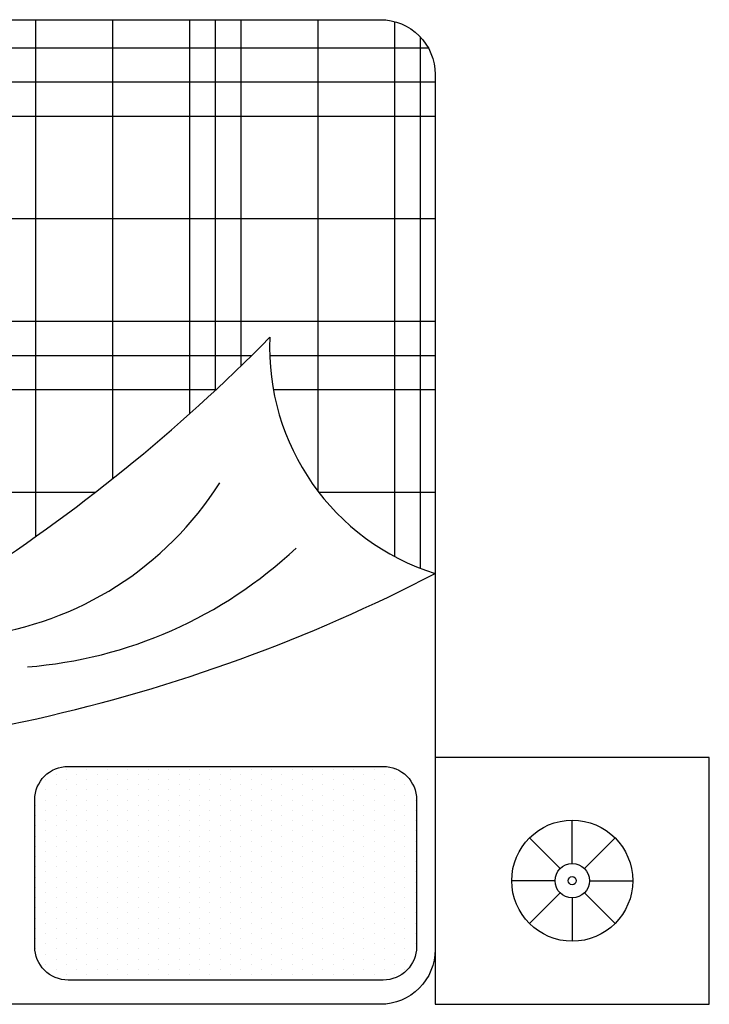
# Model space of a CAD drawing. Units: millimetres. Extents: x 2817 to 5038, y 1110 to 3565.
# Tile 21 of 21: x 4992 to 5038, y 3499 to 3565. Entities that reach past the tile are written whole.
import ezdxf

# ---------------------------------------------------------------- set-up
doc = ezdxf.new("R2010")
doc.units = ezdxf.units.MM
doc.layers.add('BLOCK', color=6, linetype='Continuous')
doc.layers.add('FURNITURE', color=219, linetype='Continuous', lineweight=18)

# ---------------------------------------------------------------- blocks, each defined once
blk = doc.blocks.new('*X7')
at = {"color": 0}
for p, q in [((276.598, 451.25), (280.51, 451.25)), ((275.455, 450.625), (280.51, 450.625)), ((274.411, 450), (280.51, 450)), ((265.51, 448.125), (267.634, 448.125)), ((271.723, 448.125), (280.51, 448.125)), ((265.51, 446.25), (268.465, 446.25)), ((269.519, 446.25), (280.51, 446.25)), ((265.51, 445.625), (268.531, 445.625)), ((268.866, 445.625), (280.51, 445.625)), ((265.51, 445), (280.51, 445)), ((265.51, 443.125), (280.51, 443.125)), ((265.51, 441.25), (280.51, 441.25)), ((265.51, 440.625), (280.51, 440.625)), ((265.634, 440), (280.386, 440))]:
    blk.add_line(p, q, dxfattribs=at)
blk = doc.blocks.new('*X8')
at = {"color": 0}
for p, q in [((280.312, 439.886), (280.312, 452.896)), ((278.906, 439.482), (278.906, 452.338)), ((277.5, 439.482), (277.5, 451.702)), ((277.031, 439.482), (277.031, 451.471)), ((276.562, 439.482), (276.562, 451.231)), ((275.156, 439.482), (275.156, 450.451)), ((265.781, 439.797), (265.781, 449.511)), ((273.75, 439.482), (273.75, 449.576)), ((266.25, 439.517), (266.25, 449.296)), ((273.281, 439.482), (273.281, 449.261)), ((272.812, 439.482), (272.812, 448.934)), ((267.656, 439.482), (267.656, 448.095)), ((271.406, 439.482), (271.406, 447.876)), ((270, 439.482), (270, 446.689)), ((269.531, 439.482), (269.531, 446.262)), ((269.062, 439.482), (269.062, 445.817))]:
    blk.add_line(p, q, dxfattribs=at)
blk = doc.blocks.new('*X9')
at = {"color": 0}
for p, q in [((266.4375, 457.03125), (266.4375, 457.03125)), ((266.8125, 457.03125), (266.8125, 457.03125)), ((267.1875, 457.03125), (267.1875, 457.03125)), ((267.5625, 457.03125), (267.5625, 457.03125)), ((267.9375, 457.03125), (267.9375, 457.03125)), ((268.3125, 457.03125), (268.3125, 457.03125)), ((268.6875, 457.03125), (268.6875, 457.03125)), ((269.0625, 457.03125), (269.0625, 457.03125)), ((269.4375, 457.03125), (269.4375, 457.03125)), ((269.8125, 457.03125), (269.8125, 457.03125)), ((270.1875, 457.03125), (270.1875, 457.03125)), ((270.5625, 457.03125), (270.5625, 457.03125)), ((270.9375, 457.03125), (270.9375, 457.03125)), ((271.3125, 457.03125), (271.3125, 457.03125)), ((271.6875, 457.03125), (271.6875, 457.03125)), ((272.0625, 457.03125), (272.0625, 457.03125)), ((266.0625, 456.84375), (266.0625, 456.84375)), ((266.25, 456.9375), (266.25, 456.9375)), ((266.4375, 456.84375), (266.4375, 456.84375)), ((266.625, 456.9375), (266.625, 456.9375)), ((266.8125, 456.84375), (266.8125, 456.84375)), ((267, 456.9375), (267, 456.9375)), ((267.1875, 456.84375), (267.1875, 456.84375)), ((267.375, 456.9375), (267.375, 456.9375)), ((267.5625, 456.84375), (267.5625, 456.84375)), ((267.75, 456.9375), (267.75, 456.9375)), ((267.9375, 456.84375), (267.9375, 456.84375)), ((268.125, 456.9375), (268.125, 456.9375)), ((268.3125, 456.84375), (268.3125, 456.84375)), ((268.5, 456.9375), (268.5, 456.9375)), ((268.6875, 456.84375), (268.6875, 456.84375)), ((268.875, 456.9375), (268.875, 456.9375)), ((269.0625, 456.84375), (269.0625, 456.84375)), ((269.25, 456.9375), (269.25, 456.9375)), ((269.4375, 456.84375), (269.4375, 456.84375)), ((269.625, 456.9375), (269.625, 456.9375)), ((269.8125, 456.84375), (269.8125, 456.84375)), ((270, 456.9375), (270, 456.9375)), ((270.1875, 456.84375), (270.1875, 456.84375)), ((270.375, 456.9375), (270.375, 456.9375)), ((270.5625, 456.84375), (270.5625, 456.84375)), ((270.75, 456.9375), (270.75, 456.9375)), ((270.9375, 456.84375), (270.9375, 456.84375)), ((271.125, 456.9375), (271.125, 456.9375)), ((271.3125, 456.84375), (271.3125, 456.84375)), ((271.5, 456.9375), (271.5, 456.9375)), ((271.6875, 456.84375), (271.6875, 456.84375)), ((271.875, 456.9375), (271.875, 456.9375)), ((272.0625, 456.84375), (272.0625, 456.84375)), ((272.25, 456.9375), (272.25, 456.9375)), ((272.4375, 456.84375), (272.4375, 456.84375)), ((266.25, 456.75), (266.25, 456.75)), ((266.625, 456.75), (266.625, 456.75)), ((267, 456.75), (267, 456.75)), ((267.375, 456.75), (267.375, 456.75)), ((267.75, 456.75), (267.75, 456.75)), ((268.125, 456.75), (268.125, 456.75)), ((268.5, 456.75), (268.5, 456.75)), ((268.875, 456.75), (268.875, 456.75)), ((269.25, 456.75), (269.25, 456.75)), ((269.625, 456.75), (269.625, 456.75)), ((270, 456.75), (270, 456.75)), ((270.375, 456.75), (270.375, 456.75)), ((270.75, 456.75), (270.75, 456.75)), ((271.125, 456.75), (271.125, 456.75)), ((271.5, 456.75), (271.5, 456.75)), ((271.875, 456.75), (271.875, 456.75)), ((272.25, 456.75), (272.25, 456.75)), ((272.625, 456.75), (272.625, 456.75)), ((265.875, 456.5625), (265.875, 456.5625)), ((266.0625, 456.65625), (266.0625, 456.65625)), ((266.25, 456.5625), (266.25, 456.5625)), ((266.4375, 456.65625), (266.4375, 456.65625)), ((266.625, 456.5625), (266.625, 456.5625)), ((266.8125, 456.65625), (266.8125, 456.65625)), ((267, 456.5625), (267, 456.5625)), ((267.1875, 456.65625), (267.1875, 456.65625)), ((267.375, 456.5625), (267.375, 456.5625)), ((267.5625, 456.65625), (267.5625, 456.65625)), ((267.75, 456.5625), (267.75, 456.5625)), ((267.9375, 456.65625), (267.9375, 456.65625)), ((268.125, 456.5625), (268.125, 456.5625)), ((268.3125, 456.65625), (268.3125, 456.65625)), ((268.5, 456.5625), (268.5, 456.5625)), ((268.6875, 456.65625), (268.6875, 456.65625)), ((268.875, 456.5625), (268.875, 456.5625)), ((269.0625, 456.65625), (269.0625, 456.65625)), ((269.25, 456.5625), (269.25, 456.5625)), ((269.4375, 456.65625), (269.4375, 456.65625)), ((269.625, 456.5625), (269.625, 456.5625)), ((269.8125, 456.65625), (269.8125, 456.65625)), ((270, 456.5625), (270, 456.5625)), ((270.1875, 456.65625), (270.1875, 456.65625)), ((270.375, 456.5625), (270.375, 456.5625)), ((270.5625, 456.65625), (270.5625, 456.65625)), ((270.75, 456.5625), (270.75, 456.5625)), ((270.9375, 456.65625), (270.9375, 456.65625)), ((271.125, 456.5625), (271.125, 456.5625)), ((271.3125, 456.65625), (271.3125, 456.65625)), ((271.5, 456.5625), (271.5, 456.5625)), ((271.6875, 456.65625), (271.6875, 456.65625)), ((271.875, 456.5625), (271.875, 456.5625)), ((272.0625, 456.65625), (272.0625, 456.65625)), ((272.25, 456.5625), (272.25, 456.5625)), ((272.4375, 456.65625), (272.4375, 456.65625)), ((272.625, 456.5625), (272.625, 456.5625)), ((265.875, 456.375), (265.875, 456.375)), ((266.0625, 456.46875), (266.0625, 456.46875)), ((266.25, 456.375), (266.25, 456.375)), ((266.4375, 456.46875), (266.4375, 456.46875)), ((266.625, 456.375), (266.625, 456.375)), ((266.8125, 456.46875), (266.8125, 456.46875)), ((267, 456.375), (267, 456.375)), ((267.1875, 456.46875), (267.1875, 456.46875)), ((267.375, 456.375), (267.375, 456.375)), ((267.5625, 456.46875), (267.5625, 456.46875)), ((267.75, 456.375), (267.75, 456.375)), ((267.9375, 456.46875), (267.9375, 456.46875)), ((268.125, 456.375), (268.125, 456.375)), ((268.3125, 456.46875), (268.3125, 456.46875)), ((268.5, 456.375), (268.5, 456.375)), ((268.6875, 456.46875), (268.6875, 456.46875)), ((268.875, 456.375), (268.875, 456.375)), ((269.0625, 456.46875), (269.0625, 456.46875)), ((269.25, 456.375), (269.25, 456.375)), ((269.4375, 456.46875), (269.4375, 456.46875)), ((269.625, 456.375), (269.625, 456.375)), ((269.8125, 456.46875), (269.8125, 456.46875)), ((270, 456.375), (270, 456.375)), ((270.1875, 456.46875), (270.1875, 456.46875)), ((270.375, 456.375), (270.375, 456.375)), ((270.5625, 456.46875), (270.5625, 456.46875)), ((270.75, 456.375), (270.75, 456.375)), ((270.9375, 456.46875), (270.9375, 456.46875)), ((271.125, 456.375), (271.125, 456.375)), ((271.3125, 456.46875), (271.3125, 456.46875)), ((271.5, 456.375), (271.5, 456.375)), ((271.6875, 456.46875), (271.6875, 456.46875)), ((271.875, 456.375), (271.875, 456.375)), ((272.0625, 456.46875), (272.0625, 456.46875)), ((272.25, 456.375), (272.25, 456.375)), ((272.4375, 456.46875), (272.4375, 456.46875)), ((272.625, 456.375), (272.625, 456.375)), ((272.8125, 456.46875), (272.8125, 456.46875)), ((265.875, 456.1875), (265.875, 456.1875)), ((266.0625, 456.28125), (266.0625, 456.28125)), ((266.25, 456.1875), (266.25, 456.1875)), ((266.4375, 456.28125), (266.4375, 456.28125)), ((266.625, 456.1875), (266.625, 456.1875)), ((266.8125, 456.28125), (266.8125, 456.28125)), ((267, 456.1875), (267, 456.1875)), ((267.1875, 456.28125), (267.1875, 456.28125)), ((267.375, 456.1875), (267.375, 456.1875)), ((267.5625, 456.28125), (267.5625, 456.28125)), ((267.75, 456.1875), (267.75, 456.1875)), ((267.9375, 456.28125), (267.9375, 456.28125)), ((268.125, 456.1875), (268.125, 456.1875)), ((268.3125, 456.28125), (268.3125, 456.28125)), ((268.5, 456.1875), (268.5, 456.1875)), ((268.6875, 456.28125), (268.6875, 456.28125)), ((268.875, 456.1875), (268.875, 456.1875)), ((269.0625, 456.28125), (269.0625, 456.28125)), ((269.25, 456.1875), (269.25, 456.1875)), ((269.4375, 456.28125), (269.4375, 456.28125)), ((269.625, 456.1875), (269.625, 456.1875)), ((269.8125, 456.28125), (269.8125, 456.28125)), ((270, 456.1875), (270, 456.1875)), ((270.1875, 456.28125), (270.1875, 456.28125)), ((270.375, 456.1875), (270.375, 456.1875)), ((270.5625, 456.28125), (270.5625, 456.28125)), ((270.75, 456.1875), (270.75, 456.1875)), ((270.9375, 456.28125), (270.9375, 456.28125)), ((271.125, 456.1875), (271.125, 456.1875)), ((271.3125, 456.28125), (271.3125, 456.28125)), ((271.5, 456.1875), (271.5, 456.1875)), ((271.6875, 456.28125), (271.6875, 456.28125)), ((271.875, 456.1875), (271.875, 456.1875)), ((272.0625, 456.28125), (272.0625, 456.28125)), ((272.25, 456.1875), (272.25, 456.1875)), ((272.4375, 456.28125), (272.4375, 456.28125)), ((272.625, 456.1875), (272.625, 456.1875)), ((272.8125, 456.28125), (272.8125, 456.28125)), ((265.875, 456), (265.875, 456)), ((266.0625, 456.09375), (266.0625, 456.09375)), ((266.25, 456), (266.25, 456)), ((266.4375, 456.09375), (266.4375, 456.09375)), ((266.625, 456), (266.625, 456)), ((266.8125, 456.09375), (266.8125, 456.09375)), ((267, 456), (267, 456)), ((267.1875, 456.09375), (267.1875, 456.09375)), ((267.375, 456), (267.375, 456)), ((267.5625, 456.09375), (267.5625, 456.09375)), ((267.75, 456), (267.75, 456)), ((267.9375, 456.09375), (267.9375, 456.09375)), ((268.125, 456), (268.125, 456)), ((268.3125, 456.09375), (268.3125, 456.09375)), ((268.5, 456), (268.5, 456)), ((268.6875, 456.09375), (268.6875, 456.09375)), ((268.875, 456), (268.875, 456)), ((269.0625, 456.09375), (269.0625, 456.09375)), ((269.25, 456), (269.25, 456)), ((269.4375, 456.09375), (269.4375, 456.09375)), ((269.625, 456), (269.625, 456)), ((269.8125, 456.09375), (269.8125, 456.09375)), ((270, 456), (270, 456)), ((270.1875, 456.09375), (270.1875, 456.09375)), ((270.375, 456), (270.375, 456)), ((270.5625, 456.09375), (270.5625, 456.09375)), ((270.75, 456), (270.75, 456)), ((270.9375, 456.09375), (270.9375, 456.09375)), ((271.125, 456), (271.125, 456)), ((271.3125, 456.09375), (271.3125, 456.09375)), ((271.5, 456), (271.5, 456)), ((271.6875, 456.09375), (271.6875, 456.09375)), ((271.875, 456), (271.875, 456)), ((272.0625, 456.09375), (272.0625, 456.09375)), ((272.25, 456), (272.25, 456)), ((272.4375, 456.09375), (272.4375, 456.09375)), ((272.625, 456), (272.625, 456)), ((272.8125, 456.09375), (272.8125, 456.09375)), ((265.875, 455.8125), (265.875, 455.8125)), ((266.0625, 455.90625), (266.0625, 455.90625)), ((266.25, 455.8125), (266.25, 455.8125)), ((266.4375, 455.90625), (266.4375, 455.90625)), ((266.625, 455.8125), (266.625, 455.8125)), ((266.8125, 455.90625), (266.8125, 455.90625)), ((267, 455.8125), (267, 455.8125)), ((267.1875, 455.90625), (267.1875, 455.90625)), ((267.375, 455.8125), (267.375, 455.8125)), ((267.5625, 455.90625), (267.5625, 455.90625)), ((267.75, 455.8125), (267.75, 455.8125)), ((267.9375, 455.90625), (267.9375, 455.90625)), ((268.125, 455.8125), (268.125, 455.8125)), ((268.3125, 455.90625), (268.3125, 455.90625)), ((268.5, 455.8125), (268.5, 455.8125)), ((268.6875, 455.90625), (268.6875, 455.90625)), ((268.875, 455.8125), (268.875, 455.8125)), ((269.0625, 455.90625), (269.0625, 455.90625)), ((269.25, 455.8125), (269.25, 455.8125)), ((269.4375, 455.90625), (269.4375, 455.90625)), ((269.625, 455.8125), (269.625, 455.8125)), ((269.8125, 455.90625), (269.8125, 455.90625)), ((270, 455.8125), (270, 455.8125)), ((270.1875, 455.90625), (270.1875, 455.90625)), ((270.375, 455.8125), (270.375, 455.8125)), ((270.5625, 455.90625), (270.5625, 455.90625)), ((270.75, 455.8125), (270.75, 455.8125)), ((270.9375, 455.90625), (270.9375, 455.90625)), ((271.125, 455.8125), (271.125, 455.8125)), ((271.3125, 455.90625), (271.3125, 455.90625)), ((271.5, 455.8125), (271.5, 455.8125)), ((271.6875, 455.90625), (271.6875, 455.90625)), ((271.875, 455.8125), (271.875, 455.8125)), ((272.0625, 455.90625), (272.0625, 455.90625)), ((272.25, 455.8125), (272.25, 455.8125)), ((272.4375, 455.90625), (272.4375, 455.90625)), ((272.625, 455.8125), (272.625, 455.8125)), ((272.8125, 455.90625), (272.8125, 455.90625)), ((265.875, 455.625), (265.875, 455.625)), ((266.0625, 455.71875), (266.0625, 455.71875)), ((266.25, 455.625), (266.25, 455.625)), ((266.4375, 455.71875), (266.4375, 455.71875)), ((266.625, 455.625), (266.625, 455.625)), ((266.8125, 455.71875), (266.8125, 455.71875)), ((267, 455.625), (267, 455.625)), ((267.1875, 455.71875), (267.1875, 455.71875)), ((267.375, 455.625), (267.375, 455.625)), ((267.5625, 455.71875), (267.5625, 455.71875)), ((267.75, 455.625), (267.75, 455.625)), ((267.9375, 455.71875), (267.9375, 455.71875)), ((268.125, 455.625), (268.125, 455.625)), ((268.3125, 455.71875), (268.3125, 455.71875)), ((268.5, 455.625), (268.5, 455.625)), ((268.6875, 455.71875), (268.6875, 455.71875)), ((268.875, 455.625), (268.875, 455.625)), ((269.0625, 455.71875), (269.0625, 455.71875)), ((269.25, 455.625), (269.25, 455.625)), ((269.4375, 455.71875), (269.4375, 455.71875)), ((269.625, 455.625), (269.625, 455.625)), ((269.8125, 455.71875), (269.8125, 455.71875)), ((270, 455.625), (270, 455.625)), ((270.1875, 455.71875), (270.1875, 455.71875)), ((270.375, 455.625), (270.375, 455.625)), ((270.5625, 455.71875), (270.5625, 455.71875)), ((270.75, 455.625), (270.75, 455.625)), ((270.9375, 455.71875), (270.9375, 455.71875)), ((271.125, 455.625), (271.125, 455.625)), ((271.3125, 455.71875), (271.3125, 455.71875)), ((271.5, 455.625), (271.5, 455.625)), ((271.6875, 455.71875), (271.6875, 455.71875)), ((271.875, 455.625), (271.875, 455.625)), ((272.0625, 455.71875), (272.0625, 455.71875)), ((272.25, 455.625), (272.25, 455.625)), ((272.4375, 455.71875), (272.4375, 455.71875)), ((272.625, 455.625), (272.625, 455.625)), ((272.8125, 455.71875), (272.8125, 455.71875)), ((265.875, 455.4375), (265.875, 455.4375)), ((266.0625, 455.53125), (266.0625, 455.53125)), ((266.25, 455.4375), (266.25, 455.4375)), ((266.4375, 455.53125), (266.4375, 455.53125)), ((266.625, 455.4375), (266.625, 455.4375)), ((266.8125, 455.53125), (266.8125, 455.53125)), ((267, 455.4375), (267, 455.4375)), ((267.1875, 455.53125), (267.1875, 455.53125)), ((267.375, 455.4375), (267.375, 455.4375)), ((267.5625, 455.53125), (267.5625, 455.53125)), ((267.75, 455.4375), (267.75, 455.4375)), ((267.9375, 455.53125), (267.9375, 455.53125)), ((268.125, 455.4375), (268.125, 455.4375)), ((268.3125, 455.53125), (268.3125, 455.53125)), ((268.5, 455.4375), (268.5, 455.4375)), ((268.6875, 455.53125), (268.6875, 455.53125)), ((268.875, 455.4375), (268.875, 455.4375)), ((269.0625, 455.53125), (269.0625, 455.53125)), ((269.25, 455.4375), (269.25, 455.4375)), ((269.4375, 455.53125), (269.4375, 455.53125)), ((269.625, 455.4375), (269.625, 455.4375)), ((269.8125, 455.53125), (269.8125, 455.53125)), ((270, 455.4375), (270, 455.4375)), ((270.1875, 455.53125), (270.1875, 455.53125)), ((270.375, 455.4375), (270.375, 455.4375)), ((270.5625, 455.53125), (270.5625, 455.53125)), ((270.75, 455.4375), (270.75, 455.4375)), ((270.9375, 455.53125), (270.9375, 455.53125)), ((271.125, 455.4375), (271.125, 455.4375)), ((271.3125, 455.53125), (271.3125, 455.53125)), ((271.5, 455.4375), (271.5, 455.4375)), ((271.6875, 455.53125), (271.6875, 455.53125)), ((271.875, 455.4375), (271.875, 455.4375)), ((272.0625, 455.53125), (272.0625, 455.53125)), ((272.25, 455.4375), (272.25, 455.4375)), ((272.4375, 455.53125), (272.4375, 455.53125)), ((272.625, 455.4375), (272.625, 455.4375)), ((272.8125, 455.53125), (272.8125, 455.53125)), ((265.875, 455.25), (265.875, 455.25)), ((266.0625, 455.34375), (266.0625, 455.34375)), ((266.25, 455.25), (266.25, 455.25)), ((266.4375, 455.34375), (266.4375, 455.34375)), ((266.625, 455.25), (266.625, 455.25)), ((266.8125, 455.34375), (266.8125, 455.34375)), ((267, 455.25), (267, 455.25)), ((267.1875, 455.34375), (267.1875, 455.34375)), ((267.375, 455.25), (267.375, 455.25)), ((267.5625, 455.34375), (267.5625, 455.34375)), ((267.75, 455.25), (267.75, 455.25)), ((267.9375, 455.34375), (267.9375, 455.34375)), ((268.125, 455.25), (268.125, 455.25)), ((268.3125, 455.34375), (268.3125, 455.34375)), ((268.5, 455.25), (268.5, 455.25)), ((268.6875, 455.34375), (268.6875, 455.34375)), ((268.875, 455.25), (268.875, 455.25)), ((269.0625, 455.34375), (269.0625, 455.34375)), ((269.25, 455.25), (269.25, 455.25)), ((269.4375, 455.34375), (269.4375, 455.34375)), ((269.625, 455.25), (269.625, 455.25)), ((269.8125, 455.34375), (269.8125, 455.34375)), ((270, 455.25), (270, 455.25)), ((270.1875, 455.34375), (270.1875, 455.34375)), ((270.375, 455.25), (270.375, 455.25)), ((270.5625, 455.34375), (270.5625, 455.34375)), ((270.75, 455.25), (270.75, 455.25)), ((270.9375, 455.34375), (270.9375, 455.34375)), ((271.125, 455.25), (271.125, 455.25)), ((271.3125, 455.34375), (271.3125, 455.34375)), ((271.5, 455.25), (271.5, 455.25)), ((271.6875, 455.34375), (271.6875, 455.34375)), ((271.875, 455.25), (271.875, 455.25)), ((272.0625, 455.34375), (272.0625, 455.34375)), ((272.25, 455.25), (272.25, 455.25)), ((272.4375, 455.34375), (272.4375, 455.34375)), ((272.625, 455.25), (272.625, 455.25)), ((272.8125, 455.34375), (272.8125, 455.34375)), ((265.875, 455.0625), (265.875, 455.0625)), ((266.0625, 455.15625), (266.0625, 455.15625)), ((266.25, 455.0625), (266.25, 455.0625)), ((266.4375, 455.15625), (266.4375, 455.15625)), ((266.625, 455.0625), (266.625, 455.0625)), ((266.8125, 455.15625), (266.8125, 455.15625)), ((267, 455.0625), (267, 455.0625)), ((267.1875, 455.15625), (267.1875, 455.15625)), ((267.375, 455.0625), (267.375, 455.0625)), ((267.5625, 455.15625), (267.5625, 455.15625)), ((267.75, 455.0625), (267.75, 455.0625)), ((267.9375, 455.15625), (267.9375, 455.15625)), ((268.125, 455.0625), (268.125, 455.0625)), ((268.3125, 455.15625), (268.3125, 455.15625)), ((268.5, 455.0625), (268.5, 455.0625)), ((268.6875, 455.15625), (268.6875, 455.15625)), ((268.875, 455.0625), (268.875, 455.0625)), ((269.0625, 455.15625), (269.0625, 455.15625)), ((269.25, 455.0625), (269.25, 455.0625)), ((269.4375, 455.15625), (269.4375, 455.15625)), ((269.625, 455.0625), (269.625, 455.0625)), ((269.8125, 455.15625), (269.8125, 455.15625)), ((270, 455.0625), (270, 455.0625)), ((270.1875, 455.15625), (270.1875, 455.15625)), ((270.375, 455.0625), (270.375, 455.0625)), ((270.5625, 455.15625), (270.5625, 455.15625)), ((270.75, 455.0625), (270.75, 455.0625)), ((270.9375, 455.15625), (270.9375, 455.15625)), ((271.125, 455.0625), (271.125, 455.0625)), ((271.3125, 455.15625), (271.3125, 455.15625)), ((271.5, 455.0625), (271.5, 455.0625)), ((271.6875, 455.15625), (271.6875, 455.15625)), ((271.875, 455.0625), (271.875, 455.0625)), ((272.0625, 455.15625), (272.0625, 455.15625)), ((272.25, 455.0625), (272.25, 455.0625)), ((272.4375, 455.15625), (272.4375, 455.15625)), ((272.625, 455.0625), (272.625, 455.0625)), ((272.8125, 455.15625), (272.8125, 455.15625)), ((265.875, 454.875), (265.875, 454.875)), ((266.0625, 454.96875), (266.0625, 454.96875)), ((266.25, 454.875), (266.25, 454.875)), ((266.4375, 454.96875), (266.4375, 454.96875)), ((266.625, 454.875), (266.625, 454.875)), ((266.8125, 454.96875), (266.8125, 454.96875)), ((267, 454.875), (267, 454.875)), ((267.1875, 454.96875), (267.1875, 454.96875)), ((267.375, 454.875), (267.375, 454.875)), ((267.5625, 454.96875), (267.5625, 454.96875)), ((267.75, 454.875), (267.75, 454.875)), ((267.9375, 454.96875), (267.9375, 454.96875)), ((268.125, 454.875), (268.125, 454.875)), ((268.3125, 454.96875), (268.3125, 454.96875)), ((268.5, 454.875), (268.5, 454.875)), ((268.6875, 454.96875), (268.6875, 454.96875)), ((268.875, 454.875), (268.875, 454.875)), ((269.0625, 454.96875), (269.0625, 454.96875)), ((269.25, 454.875), (269.25, 454.875)), ((269.4375, 454.96875), (269.4375, 454.96875)), ((269.625, 454.875), (269.625, 454.875)), ((269.8125, 454.96875), (269.8125, 454.96875)), ((270, 454.875), (270, 454.875)), ((270.1875, 454.96875), (270.1875, 454.96875)), ((270.375, 454.875), (270.375, 454.875)), ((270.5625, 454.96875), (270.5625, 454.96875)), ((270.75, 454.875), (270.75, 454.875)), ((270.9375, 454.96875), (270.9375, 454.96875)), ((271.125, 454.875), (271.125, 454.875)), ((271.3125, 454.96875), (271.3125, 454.96875)), ((271.5, 454.875), (271.5, 454.875)), ((271.6875, 454.96875), (271.6875, 454.96875)), ((271.875, 454.875), (271.875, 454.875)), ((272.0625, 454.96875), (272.0625, 454.96875)), ((272.25, 454.875), (272.25, 454.875)), ((272.4375, 454.96875), (272.4375, 454.96875)), ((272.625, 454.875), (272.625, 454.875)), ((272.8125, 454.96875), (272.8125, 454.96875)), ((265.875, 454.6875), (265.875, 454.6875)), ((266.0625, 454.78125), (266.0625, 454.78125)), ((266.25, 454.6875), (266.25, 454.6875)), ((266.4375, 454.78125), (266.4375, 454.78125)), ((266.625, 454.6875), (266.625, 454.6875)), ((266.8125, 454.78125), (266.8125, 454.78125)), ((267, 454.6875), (267, 454.6875)), ((267.1875, 454.78125), (267.1875, 454.78125)), ((267.375, 454.6875), (267.375, 454.6875)), ((267.5625, 454.78125), (267.5625, 454.78125)), ((267.75, 454.6875), (267.75, 454.6875)), ((267.9375, 454.78125), (267.9375, 454.78125)), ((268.125, 454.6875), (268.125, 454.6875)), ((268.3125, 454.78125), (268.3125, 454.78125)), ((268.5, 454.6875), (268.5, 454.6875)), ((268.6875, 454.78125), (268.6875, 454.78125)), ((268.875, 454.6875), (268.875, 454.6875)), ((269.0625, 454.78125), (269.0625, 454.78125)), ((269.25, 454.6875), (269.25, 454.6875)), ((269.4375, 454.78125), (269.4375, 454.78125)), ((269.625, 454.6875), (269.625, 454.6875)), ((269.8125, 454.78125), (269.8125, 454.78125)), ((270, 454.6875), (270, 454.6875)), ((270.1875, 454.78125), (270.1875, 454.78125)), ((270.375, 454.6875), (270.375, 454.6875)), ((270.5625, 454.78125), (270.5625, 454.78125)), ((270.75, 454.6875), (270.75, 454.6875)), ((270.9375, 454.78125), (270.9375, 454.78125)), ((271.125, 454.6875), (271.125, 454.6875)), ((271.3125, 454.78125), (271.3125, 454.78125)), ((271.5, 454.6875), (271.5, 454.6875)), ((271.6875, 454.78125), (271.6875, 454.78125)), ((271.875, 454.6875), (271.875, 454.6875)), ((272.0625, 454.78125), (272.0625, 454.78125)), ((272.25, 454.6875), (272.25, 454.6875)), ((272.4375, 454.78125), (272.4375, 454.78125)), ((272.625, 454.6875), (272.625, 454.6875)), ((272.8125, 454.78125), (272.8125, 454.78125)), ((266.0625, 454.59375), (266.0625, 454.59375)), ((266.4375, 454.59375), (266.4375, 454.59375)), ((266.8125, 454.59375), (266.8125, 454.59375)), ((267.1875, 454.59375), (267.1875, 454.59375)), ((267.5625, 454.59375), (267.5625, 454.59375)), ((267.9375, 454.59375), (267.9375, 454.59375)), ((268.3125, 454.59375), (268.3125, 454.59375)), ((268.6875, 454.59375), (268.6875, 454.59375)), ((269.0625, 454.59375), (269.0625, 454.59375)), ((269.4375, 454.59375), (269.4375, 454.59375)), ((269.8125, 454.59375), (269.8125, 454.59375)), ((270.1875, 454.59375), (270.1875, 454.59375)), ((270.5625, 454.59375), (270.5625, 454.59375)), ((270.9375, 454.59375), (270.9375, 454.59375)), ((271.3125, 454.59375), (271.3125, 454.59375)), ((271.6875, 454.59375), (271.6875, 454.59375)), ((272.0625, 454.59375), (272.0625, 454.59375)), ((272.4375, 454.59375), (272.4375, 454.59375)), ((272.8125, 454.59375), (272.8125, 454.59375)), ((265.875, 454.5), (265.875, 454.5)), ((266.0625, 454.40625), (266.0625, 454.40625)), ((266.25, 454.5), (266.25, 454.5)), ((266.4375, 454.40625), (266.4375, 454.40625)), ((266.625, 454.5), (266.625, 454.5)), ((266.8125, 454.40625), (266.8125, 454.40625)), ((267, 454.5), (267, 454.5)), ((267.1875, 454.40625), (267.1875, 454.40625)), ((267.375, 454.5), (267.375, 454.5)), ((267.5625, 454.40625), (267.5625, 454.40625)), ((267.75, 454.5), (267.75, 454.5)), ((267.9375, 454.40625), (267.9375, 454.40625)), ((268.125, 454.5), (268.125, 454.5)), ((268.3125, 454.40625), (268.3125, 454.40625)), ((268.5, 454.5), (268.5, 454.5)), ((268.6875, 454.40625), (268.6875, 454.40625)), ((268.875, 454.5), (268.875, 454.5)), ((269.0625, 454.40625), (269.0625, 454.40625)), ((269.25, 454.5), (269.25, 454.5)), ((269.4375, 454.40625), (269.4375, 454.40625)), ((269.625, 454.5), (269.625, 454.5)), ((269.8125, 454.40625), (269.8125, 454.40625)), ((270, 454.5), (270, 454.5)), ((270.1875, 454.40625), (270.1875, 454.40625)), ((270.375, 454.5), (270.375, 454.5)), ((270.5625, 454.40625), (270.5625, 454.40625)), ((270.75, 454.5), (270.75, 454.5)), ((270.9375, 454.40625), (270.9375, 454.40625)), ((271.125, 454.5), (271.125, 454.5)), ((271.3125, 454.40625), (271.3125, 454.40625)), ((271.5, 454.5), (271.5, 454.5)), ((271.6875, 454.40625), (271.6875, 454.40625)), ((271.875, 454.5), (271.875, 454.5)), ((272.0625, 454.40625), (272.0625, 454.40625)), ((272.25, 454.5), (272.25, 454.5)), ((272.4375, 454.40625), (272.4375, 454.40625)), ((272.625, 454.5), (272.625, 454.5)), ((272.8125, 454.40625), (272.8125, 454.40625)), ((265.875, 454.3125), (265.875, 454.3125)), ((266.0625, 454.21875), (266.0625, 454.21875)), ((266.25, 454.3125), (266.25, 454.3125)), ((266.4375, 454.21875), (266.4375, 454.21875)), ((266.625, 454.3125), (266.625, 454.3125)), ((266.8125, 454.21875), (266.8125, 454.21875)), ((267, 454.3125), (267, 454.3125)), ((267.1875, 454.21875), (267.1875, 454.21875)), ((267.375, 454.3125), (267.375, 454.3125)), ((267.5625, 454.21875), (267.5625, 454.21875)), ((267.75, 454.3125), (267.75, 454.3125)), ((267.9375, 454.21875), (267.9375, 454.21875)), ((268.125, 454.3125), (268.125, 454.3125)), ((268.3125, 454.21875), (268.3125, 454.21875)), ((268.5, 454.3125), (268.5, 454.3125)), ((268.6875, 454.21875), (268.6875, 454.21875)), ((268.875, 454.3125), (268.875, 454.3125)), ((269.0625, 454.21875), (269.0625, 454.21875)), ((269.25, 454.3125), (269.25, 454.3125)), ((269.4375, 454.21875), (269.4375, 454.21875)), ((269.625, 454.3125), (269.625, 454.3125)), ((269.8125, 454.21875), (269.8125, 454.21875)), ((270, 454.3125), (270, 454.3125)), ((270.1875, 454.21875), (270.1875, 454.21875)), ((270.375, 454.3125), (270.375, 454.3125)), ((270.5625, 454.21875), (270.5625, 454.21875)), ((270.75, 454.3125), (270.75, 454.3125)), ((270.9375, 454.21875), (270.9375, 454.21875)), ((271.125, 454.3125), (271.125, 454.3125)), ((271.3125, 454.21875), (271.3125, 454.21875)), ((271.5, 454.3125), (271.5, 454.3125)), ((271.6875, 454.21875), (271.6875, 454.21875)), ((271.875, 454.3125), (271.875, 454.3125)), ((272.0625, 454.21875), (272.0625, 454.21875)), ((272.25, 454.3125), (272.25, 454.3125)), ((272.4375, 454.21875), (272.4375, 454.21875)), ((272.625, 454.3125), (272.625, 454.3125)), ((272.8125, 454.21875), (272.8125, 454.21875)), ((265.875, 454.125), (265.875, 454.125)), ((266.0625, 454.03125), (266.0625, 454.03125)), ((266.25, 454.125), (266.25, 454.125)), ((266.4375, 454.03125), (266.4375, 454.03125)), ((266.625, 454.125), (266.625, 454.125)), ((266.8125, 454.03125), (266.8125, 454.03125)), ((267, 454.125), (267, 454.125)), ((267.1875, 454.03125), (267.1875, 454.03125)), ((267.375, 454.125), (267.375, 454.125)), ((267.5625, 454.03125), (267.5625, 454.03125)), ((267.75, 454.125), (267.75, 454.125)), ((267.9375, 454.03125), (267.9375, 454.03125)), ((268.125, 454.125), (268.125, 454.125)), ((268.3125, 454.03125), (268.3125, 454.03125)), ((268.5, 454.125), (268.5, 454.125)), ((268.6875, 454.03125), (268.6875, 454.03125)), ((268.875, 454.125), (268.875, 454.125)), ((269.0625, 454.03125), (269.0625, 454.03125)), ((269.25, 454.125), (269.25, 454.125)), ((269.4375, 454.03125), (269.4375, 454.03125)), ((269.625, 454.125), (269.625, 454.125)), ((269.8125, 454.03125), (269.8125, 454.03125)), ((270, 454.125), (270, 454.125)), ((270.1875, 454.03125), (270.1875, 454.03125)), ((270.375, 454.125), (270.375, 454.125)), ((270.5625, 454.03125), (270.5625, 454.03125)), ((270.75, 454.125), (270.75, 454.125)), ((270.9375, 454.03125), (270.9375, 454.03125)), ((271.125, 454.125), (271.125, 454.125)), ((271.3125, 454.03125), (271.3125, 454.03125)), ((271.5, 454.125), (271.5, 454.125)), ((271.6875, 454.03125), (271.6875, 454.03125)), ((271.875, 454.125), (271.875, 454.125)), ((272.0625, 454.03125), (272.0625, 454.03125)), ((272.25, 454.125), (272.25, 454.125)), ((272.4375, 454.03125), (272.4375, 454.03125)), ((272.625, 454.125), (272.625, 454.125)), ((272.8125, 454.03125), (272.8125, 454.03125)), ((265.875, 453.9375), (265.875, 453.9375)), ((266.0625, 453.84375), (266.0625, 453.84375)), ((266.25, 453.9375), (266.25, 453.9375)), ((266.4375, 453.84375), (266.4375, 453.84375)), ((266.625, 453.9375), (266.625, 453.9375)), ((266.8125, 453.84375), (266.8125, 453.84375)), ((267, 453.9375), (267, 453.9375)), ((267.1875, 453.84375), (267.1875, 453.84375)), ((267.375, 453.9375), (267.375, 453.9375)), ((267.5625, 453.84375), (267.5625, 453.84375)), ((267.75, 453.9375), (267.75, 453.9375)), ((267.9375, 453.84375), (267.9375, 453.84375)), ((268.125, 453.9375), (268.125, 453.9375)), ((268.3125, 453.84375), (268.3125, 453.84375)), ((268.5, 453.9375), (268.5, 453.9375)), ((268.6875, 453.84375), (268.6875, 453.84375)), ((268.875, 453.9375), (268.875, 453.9375)), ((269.0625, 453.84375), (269.0625, 453.84375)), ((269.25, 453.9375), (269.25, 453.9375)), ((269.4375, 453.84375), (269.4375, 453.84375)), ((269.625, 453.9375), (269.625, 453.9375)), ((269.8125, 453.84375), (269.8125, 453.84375)), ((270, 453.9375), (270, 453.9375)), ((270.1875, 453.84375), (270.1875, 453.84375)), ((270.375, 453.9375), (270.375, 453.9375)), ((270.5625, 453.84375), (270.5625, 453.84375)), ((270.75, 453.9375), (270.75, 453.9375)), ((270.9375, 453.84375), (270.9375, 453.84375)), ((271.125, 453.9375), (271.125, 453.9375)), ((271.3125, 453.84375), (271.3125, 453.84375)), ((271.5, 453.9375), (271.5, 453.9375)), ((271.6875, 453.84375), (271.6875, 453.84375)), ((271.875, 453.9375), (271.875, 453.9375)), ((272.0625, 453.84375), (272.0625, 453.84375)), ((272.25, 453.9375), (272.25, 453.9375)), ((272.4375, 453.84375), (272.4375, 453.84375)), ((272.625, 453.9375), (272.625, 453.9375)), ((272.8125, 453.84375), (272.8125, 453.84375)), ((265.875, 453.75), (265.875, 453.75)), ((266.0625, 453.65625), (266.0625, 453.65625)), ((266.25, 453.75), (266.25, 453.75)), ((266.4375, 453.65625), (266.4375, 453.65625)), ((266.625, 453.75), (266.625, 453.75)), ((266.8125, 453.65625), (266.8125, 453.65625)), ((267, 453.75), (267, 453.75)), ((267.1875, 453.65625), (267.1875, 453.65625)), ((267.375, 453.75), (267.375, 453.75)), ((267.5625, 453.65625), (267.5625, 453.65625)), ((267.75, 453.75), (267.75, 453.75)), ((267.9375, 453.65625), (267.9375, 453.65625)), ((268.125, 453.75), (268.125, 453.75)), ((268.3125, 453.65625), (268.3125, 453.65625)), ((268.5, 453.75), (268.5, 453.75)), ((268.6875, 453.65625), (268.6875, 453.65625)), ((268.875, 453.75), (268.875, 453.75)), ((269.0625, 453.65625), (269.0625, 453.65625)), ((269.25, 453.75), (269.25, 453.75)), ((269.4375, 453.65625), (269.4375, 453.65625)), ((269.625, 453.75), (269.625, 453.75)), ((269.8125, 453.65625), (269.8125, 453.65625)), ((270, 453.75), (270, 453.75)), ((270.1875, 453.65625), (270.1875, 453.65625)), ((270.375, 453.75), (270.375, 453.75)), ((270.5625, 453.65625), (270.5625, 453.65625)), ((270.75, 453.75), (270.75, 453.75)), ((270.9375, 453.65625), (270.9375, 453.65625)), ((271.125, 453.75), (271.125, 453.75)), ((271.3125, 453.65625), (271.3125, 453.65625)), ((271.5, 453.75), (271.5, 453.75)), ((271.6875, 453.65625), (271.6875, 453.65625)), ((271.875, 453.75), (271.875, 453.75)), ((272.0625, 453.65625), (272.0625, 453.65625)), ((272.25, 453.75), (272.25, 453.75)), ((272.4375, 453.65625), (272.4375, 453.65625)), ((272.625, 453.75), (272.625, 453.75)), ((272.8125, 453.65625), (272.8125, 453.65625)), ((266.0625, 453.46875), (266.0625, 453.46875)), ((266.25, 453.5625), (266.25, 453.5625)), ((266.4375, 453.46875), (266.4375, 453.46875)), ((266.625, 453.5625), (266.625, 453.5625)), ((266.8125, 453.46875), (266.8125, 453.46875)), ((267, 453.5625), (267, 453.5625)), ((267.1875, 453.46875), (267.1875, 453.46875)), ((267.375, 453.5625), (267.375, 453.5625)), ((267.5625, 453.46875), (267.5625, 453.46875)), ((267.75, 453.5625), (267.75, 453.5625)), ((267.9375, 453.46875), (267.9375, 453.46875)), ((268.125, 453.5625), (268.125, 453.5625)), ((268.3125, 453.46875), (268.3125, 453.46875)), ((268.5, 453.5625), (268.5, 453.5625)), ((268.6875, 453.46875), (268.6875, 453.46875)), ((268.875, 453.5625), (268.875, 453.5625)), ((269.0625, 453.46875), (269.0625, 453.46875)), ((269.25, 453.5625), (269.25, 453.5625)), ((269.4375, 453.46875), (269.4375, 453.46875)), ((269.625, 453.5625), (269.625, 453.5625)), ((269.8125, 453.46875), (269.8125, 453.46875)), ((270, 453.5625), (270, 453.5625)), ((270.1875, 453.46875), (270.1875, 453.46875)), ((270.375, 453.5625), (270.375, 453.5625)), ((270.5625, 453.46875), (270.5625, 453.46875)), ((270.75, 453.5625), (270.75, 453.5625)), ((270.9375, 453.46875), (270.9375, 453.46875)), ((271.125, 453.5625), (271.125, 453.5625)), ((271.3125, 453.46875), (271.3125, 453.46875)), ((271.5, 453.5625), (271.5, 453.5625)), ((271.6875, 453.46875), (271.6875, 453.46875)), ((271.875, 453.5625), (271.875, 453.5625)), ((272.0625, 453.46875), (272.0625, 453.46875)), ((272.25, 453.5625), (272.25, 453.5625)), ((272.4375, 453.46875), (272.4375, 453.46875)), ((272.625, 453.5625), (272.625, 453.5625)), ((266.0625, 453.28125), (266.0625, 453.28125)), ((266.25, 453.375), (266.25, 453.375)), ((266.4375, 453.28125), (266.4375, 453.28125)), ((266.625, 453.375), (266.625, 453.375)), ((266.8125, 453.28125), (266.8125, 453.28125)), ((267, 453.375), (267, 453.375)), ((267.1875, 453.28125), (267.1875, 453.28125)), ((267.375, 453.375), (267.375, 453.375)), ((267.5625, 453.28125), (267.5625, 453.28125)), ((267.75, 453.375), (267.75, 453.375)), ((267.9375, 453.28125), (267.9375, 453.28125)), ((268.125, 453.375), (268.125, 453.375)), ((268.3125, 453.28125), (268.3125, 453.28125)), ((268.5, 453.375), (268.5, 453.375)), ((268.6875, 453.28125), (268.6875, 453.28125)), ((268.875, 453.375), (268.875, 453.375)), ((269.0625, 453.28125), (269.0625, 453.28125)), ((269.25, 453.375), (269.25, 453.375)), ((269.4375, 453.28125), (269.4375, 453.28125)), ((269.625, 453.375), (269.625, 453.375)), ((269.8125, 453.28125), (269.8125, 453.28125)), ((270, 453.375), (270, 453.375)), ((270.1875, 453.28125), (270.1875, 453.28125)), ((270.375, 453.375), (270.375, 453.375)), ((270.5625, 453.28125), (270.5625, 453.28125)), ((270.75, 453.375), (270.75, 453.375)), ((270.9375, 453.28125), (270.9375, 453.28125)), ((271.125, 453.375), (271.125, 453.375)), ((271.3125, 453.28125), (271.3125, 453.28125)), ((271.5, 453.375), (271.5, 453.375)), ((271.6875, 453.28125), (271.6875, 453.28125)), ((271.875, 453.375), (271.875, 453.375)), ((272.0625, 453.28125), (272.0625, 453.28125)), ((272.25, 453.375), (272.25, 453.375)), ((272.4375, 453.28125), (272.4375, 453.28125)), ((272.625, 453.375), (272.625, 453.375)), ((266.25, 453.1875), (266.25, 453.1875)), ((266.625, 453.1875), (266.625, 453.1875)), ((267, 453.1875), (267, 453.1875)), ((267.375, 453.1875), (267.375, 453.1875)), ((267.75, 453.1875), (267.75, 453.1875)), ((268.125, 453.1875), (268.125, 453.1875)), ((268.5, 453.1875), (268.5, 453.1875)), ((268.875, 453.1875), (268.875, 453.1875)), ((269.25, 453.1875), (269.25, 453.1875)), ((269.625, 453.1875), (269.625, 453.1875)), ((270, 453.1875), (270, 453.1875)), ((270.375, 453.1875), (270.375, 453.1875)), ((270.75, 453.1875), (270.75, 453.1875)), ((271.125, 453.1875), (271.125, 453.1875)), ((271.5, 453.1875), (271.5, 453.1875)), ((271.875, 453.1875), (271.875, 453.1875)), ((272.25, 453.1875), (272.25, 453.1875))]:
    blk.add_line(p, q, dxfattribs=at)
blk = doc.blocks.new('A$C52E67D0D')
at = {"layer": 'BLOCK'}
for p, q in [((250.5, 1605.5), (250.5, 1684.7)), ((228.3, 1596.3), (172.3, 1652.3)), ((272.7, 1596.3), (328.7, 1652.3)), ((219.1, 1574.1), (139.9, 1574.1)), ((281.9, 1574.1), (361.1, 1574.1)), ((228.3, 1551.9), (172.3, 1495.9)), ((272.7, 1551.9), (328.7, 1495.9)), ((250.5, 1542.8), (250.5, 1463.5))]:
    blk.add_line(p, q, dxfattribs=at)
for points in [[(1901, 0), (601, 0, -0.414214), (501, 100), (501, 1700, -0.414214), (601, 1800), (1901, 1800, -0.414214), (2001, 1700), (2001, 100, -0.414214)], [(1171.8, 1365.1), (595.8, 1365.1, -0.414214), (535, 1425.9), (535, 1694.8, -0.414214), (595.8, 1755.7), (1171.8, 1755.7, -0.414214), (1232.6, 1694.8), (1232.6, 1425.9, -0.414214)]]:
    blk.add_lwpolyline(points, format="xyb", close=True, dxfattribs=at)
blk.add_lwpolyline([(501, 1348.6), (501, 1799.6), (0, 1799.6), (0, 1348.6)], close=True, dxfattribs=at)
for radius in [110.6, 31.4, 7.46]:
    blk.add_circle((250.5, 1574.1), radius, dxfattribs=at)
for centre, radius, start, end in [((1888.6, -1664.5), 3015.3, 87.8642, 117.4001), ((3101, -1685.8), 3227.7, 109.926, 135.3977), ((1308.8, 377.9), 807.6, 94.4436, 133.2788), ((1410.8, 520.2), 610.8, 97.2157, 147.6656), ((371.4, 600.4), 432, 357.3792, 72.5379)]:
    blk.add_arc(centre, radius, start, end, dxfattribs=at)
at = {"layer": 'BLOCK', "xscale": 100, "yscale": 100, "zscale": 100}
for name in ['*X9', '*X8', '*X7']:
    blk.add_blockref(name, (-26050, -43948.2), dxfattribs=at)

msp = doc.modelspace()

# ---------------------------------------------------------------- block references
at = {"layer": 'FURNITURE', "xscale": 0.0367705835331598, "yscale": 0.0367705835331598, "zscale": 0.0367705835331598, "rotation": 180}
msp.add_blockref('A$C52E67D0D', (5038.0262, 3565.4526), dxfattribs=at)

doc.saveas('drawing.dxf')
